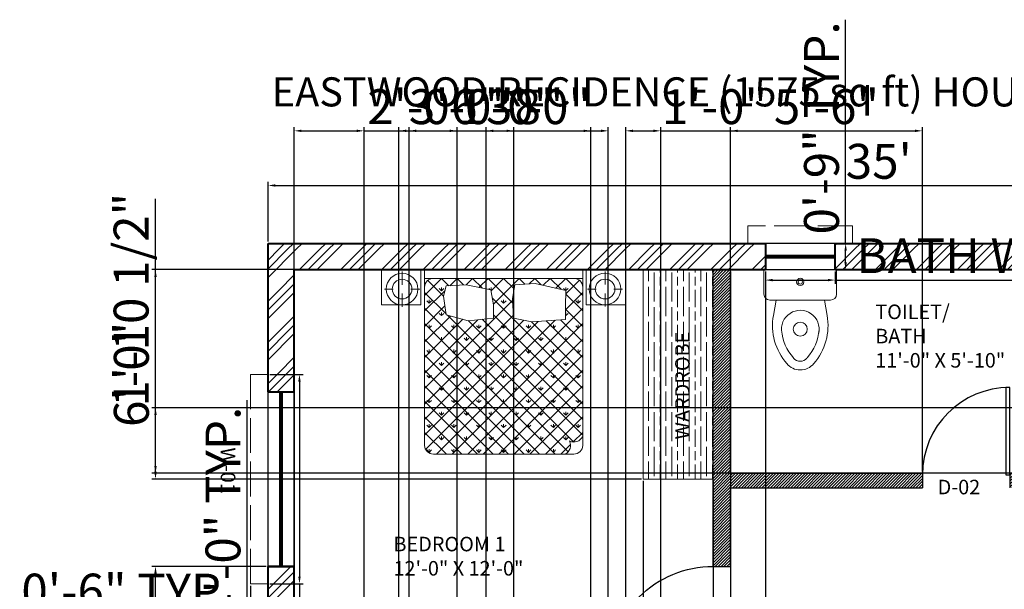
# Model space of a CAD drawing. Units: inches. Extents: x 2386 to 3029, y 792 to 1465.
# Tile 10 of 12: x 2386 to 2724, y 1269 to 1465. Entities that reach past the tile are written whole.
import ezdxf

# ---------------------------------------------------------------- set-up
doc = ezdxf.new("R2010")
doc.units = ezdxf.units.IN
doc.linetypes.add('ACAD_ISO02W100', pattern=[15, 12, -3])
for name, color, linetype, lineweight in [('A-AREA-IDEN', 4, 'Continuous', 25), ('A-DIMS', 1, 'Continuous', 18), ('A-DOOR', 2, 'Continuous', 25), ('A-FLOR-CASE', 6, 'Continuous', 18), ('A-FLOR-CASE-PATT', 9, 'Continuous', 13), ('A-FLOR-FIXT', 9, 'Continuous', 18), ('A-FURN', 6, 'Continuous', 18), ('A-TEXT', 4, 'Continuous', 25), ('A-WALL-EXT', 7, 'Continuous', 40), ('A-WALL-INT', 9, 'Continuous', 30), ('A-WALL-PATT', 9, 'Continuous', 13), ('A-WINDOW', 4, 'Continuous', 25), ('A-WINDOW-OVHD', 4, 'ACAD_ISO02W100', 18)]:
    doc.layers.add(name, color=color, linetype=linetype, lineweight=lineweight)
doc.styles.get("Standard").update_dxf_attribs({"font": 'arial.ttf'})
doc.dimstyles.new('ISO-25', dxfattribs={"dimtxt": 12, "dimasz": 2.5, "dimexe": 1.25, "dimexo": 0.625, "dimtad": 1, "dimlunit": 4, "dimtxsty": 'Standard', "dimcen": 2.5, "dimadec": 0, "dimazin": 0, "dimtfac": 1, "dimtmove": 0, "dimatfit": 3, "dimfxl": 1, "dimarcsym": 0})

# ---------------------------------------------------------------- blocks, each defined once
blk = doc.blocks.new('*X5')
at = {"color": 0}
for p, q in [((0, 0), (0, 0)), ((-707, -141), (-707, -104)), ((-566, 0), (-566, 0)), ((-566, 0), (-566, 0)), ((-283, 0), (-283, 0)), ((-283, 0), (-283, 0)), ((-141, -141), (-141, -104)), ((283, 0), (283, 0)), ((566, 0), (566, 0)), ((707, -135), (707, -104)), ((-707, -141), (-734, -115)), ((-707, -141), (-681, -115)), ((-156, -126), (-168, -115)), ((-141, -141), (-142, -140)), ((-141, -141), (-115, -115)), ((120, -120), (115, -115)), ((699, -134), (681, -115)), ((710, -139), (734, -115)), ((-849, -283), (-875, -256)), ((-849, -283), (-849, -245)), ((-849, -283), (-822, -256)), ((0, -283), (-27, -256)), ((0, -283), (0, -245)), ((0, -283), (27, -256)), ((849, -283), (822, -256)), ((849, -283), (849, -245)), ((849, -283), (875, -256)), ((-707, -424), (-734, -398)), ((-707, -424), (-707, -387)), ((-707, -424), (-681, -398)), ((-116, -399), (-115, -398)), ((707, -424), (703, -420)), ((707, -424), (707, -387)), ((707, -424), (734, -398)), ((-849, -566), (-875, -539)), ((-849, -566), (-849, -528)), ((-849, -566), (-822, -539)), ((-566, -566), (-592, -539)), ((-566, -566), (-566, -528)), ((-566, -566), (-539, -539)), ((-283, -566), (-309, -539)), ((-283, -566), (-283, -528)), ((-283, -566), (-256, -539)), ((0, -566), (-27, -539)), ((0, -566), (0, -528)), ((0, -566), (27, -539)), ((283, -566), (256, -539)), ((283, -566), (283, -528)), ((283, -566), (309, -539)), ((566, -566), (539, -539)), ((566, -566), (566, -528)), ((566, -566), (592, -539)), ((849, -566), (822, -539)), ((849, -566), (849, -528)), ((849, -566), (875, -539)), ((-707, -707), (-707, -670)), ((-424, -707), (-424, -670)), ((-141, -707), (-141, -670)), ((141, -707), (141, -670)), ((424, -707), (424, -670)), ((707, -707), (707, -670)), ((-707, -707), (-734, -681)), ((-707, -707), (-681, -681)), ((-424, -707), (-451, -681)), ((-424, -707), (-398, -681)), ((-141, -707), (-168, -681)), ((-141, -707), (-115, -681)), ((141, -707), (115, -681)), ((141, -707), (168, -681)), ((424, -707), (398, -681)), ((424, -707), (451, -681)), ((707, -707), (681, -681)), ((707, -707), (734, -681)), ((-849, -849), (-875, -822)), ((-849, -849), (-849, -811)), ((-849, -849), (-822, -822)), ((-566, -849), (-592, -822)), ((-566, -849), (-566, -811)), ((-566, -849), (-539, -822)), ((-283, -849), (-309, -822)), ((-283, -849), (-283, -811)), ((-283, -849), (-256, -822)), ((0, -849), (-27, -822)), ((0, -849), (0, -811)), ((0, -849), (27, -822)), ((283, -849), (256, -822)), ((283, -849), (283, -811)), ((283, -849), (309, -822)), ((566, -849), (539, -822)), ((566, -849), (566, -811)), ((566, -849), (592, -822)), ((849, -849), (822, -822)), ((849, -849), (849, -811)), ((849, -849), (875, -822)), ((-707, -990), (-734, -963)), ((-707, -990), (-707, -952)), ((-707, -990), (-681, -963)), ((-424, -990), (-451, -963)), ((-424, -990), (-424, -952)), ((-424, -990), (-398, -963)), ((-141, -990), (-168, -963)), ((-141, -990), (-141, -952)), ((-141, -990), (-115, -963)), ((141, -990), (115, -963)), ((141, -990), (141, -952)), ((141, -990), (168, -963)), ((424, -990), (398, -963)), ((424, -990), (424, -952)), ((424, -990), (451, -963)), ((707, -990), (681, -963)), ((707, -990), (707, -952)), ((707, -990), (734, -963)), ((-849, -1131), (-875, -1105)), ((-849, -1131), (-849, -1094)), ((-849, -1131), (-822, -1105)), ((-566, -1131), (-592, -1105)), ((-566, -1131), (-566, -1094)), ((-566, -1131), (-539, -1105)), ((-283, -1131), (-309, -1105)), ((-283, -1131), (-283, -1094)), ((-283, -1131), (-256, -1105)), ((0, -1131), (-27, -1105)), ((0, -1131), (0, -1094)), ((0, -1131), (27, -1105)), ((283, -1131), (256, -1105)), ((283, -1131), (283, -1094)), ((283, -1131), (309, -1105)), ((566, -1131), (539, -1105)), ((566, -1131), (566, -1094)), ((566, -1131), (592, -1105)), ((849, -1131), (822, -1105)), ((849, -1131), (849, -1094)), ((849, -1131), (875, -1105)), ((-707, -1273), (-734, -1246)), ((-707, -1273), (-707, -1235)), ((-707, -1273), (-681, -1246)), ((-424, -1273), (-451, -1246)), ((-424, -1273), (-424, -1235)), ((-424, -1273), (-398, -1246)), ((-141, -1273), (-168, -1246)), ((-141, -1273), (-141, -1235)), ((-141, -1273), (-115, -1246)), ((141, -1273), (115, -1246)), ((141, -1273), (141, -1235)), ((141, -1273), (168, -1246)), ((424, -1273), (398, -1246)), ((424, -1273), (424, -1235)), ((424, -1273), (451, -1246)), ((707, -1273), (681, -1246)), ((707, -1273), (707, -1235)), ((707, -1273), (734, -1246)), ((-849, -1414), (-875, -1388)), ((-849, -1414), (-849, -1377)), ((-849, -1414), (-822, -1388)), ((-566, -1414), (-592, -1388)), ((-566, -1414), (-566, -1377)), ((-566, -1414), (-539, -1388)), ((-283, -1414), (-309, -1388)), ((-283, -1414), (-283, -1377)), ((-283, -1414), (-256, -1388)), ((0, -1414), (-27, -1388)), ((0, -1414), (0, -1377)), ((0, -1414), (27, -1388)), ((283, -1414), (256, -1388)), ((283, -1414), (283, -1377)), ((283, -1414), (309, -1388)), ((566, -1414), (539, -1388)), ((566, -1414), (566, -1377)), ((566, -1414), (592, -1388)), ((849, -1414), (822, -1388)), ((849, -1414), (849, -1377)), ((849, -1414), (875, -1388)), ((-707, -1556), (-734, -1529)), ((-707, -1556), (-707, -1518)), ((-707, -1556), (-681, -1529)), ((-424, -1556), (-451, -1529)), ((-424, -1556), (-424, -1518)), ((-424, -1556), (-398, -1529)), ((-141, -1556), (-168, -1529)), ((-141, -1556), (-141, -1518)), ((-141, -1556), (-115, -1529)), ((141, -1556), (115, -1529)), ((141, -1556), (141, -1518)), ((141, -1556), (168, -1529)), ((424, -1556), (398, -1529)), ((424, -1556), (424, -1518)), ((424, -1556), (451, -1529)), ((707, -1556), (681, -1529)), ((707, -1556), (707, -1518)), ((707, -1556), (734, -1529)), ((-849, -1697), (-875, -1671)), ((-849, -1697), (-849, -1660)), ((-849, -1697), (-822, -1671)), ((-566, -1697), (-592, -1671)), ((-566, -1697), (-566, -1660)), ((-566, -1697), (-539, -1671)), ((-283, -1697), (-309, -1671)), ((-283, -1697), (-283, -1660)), ((-283, -1697), (-256, -1671)), ((0, -1697), (-27, -1671)), ((0, -1697), (0, -1660)), ((0, -1697), (27, -1671)), ((283, -1697), (256, -1671)), ((283, -1697), (283, -1660)), ((283, -1697), (309, -1671)), ((566, -1697), (539, -1671)), ((566, -1697), (566, -1660)), ((566, -1697), (592, -1671)), ((849, -1697), (822, -1671)), ((849, -1697), (849, -1660)), ((849, -1697), (875, -1671)), ((-707, -1838), (-734, -1812)), ((-707, -1838), (-707, -1801)), ((-707, -1838), (-681, -1812)), ((-424, -1838), (-451, -1812)), ((-424, -1838), (-424, -1801)), ((-424, -1838), (-398, -1812)), ((-141, -1838), (-168, -1812)), ((-141, -1838), (-141, -1801)), ((-141, -1838), (-115, -1812)), ((141, -1838), (115, -1812)), ((141, -1838), (141, -1801)), ((141, -1838), (168, -1812)), ((424, -1838), (398, -1812)), ((424, -1838), (424, -1801)), ((424, -1838), (451, -1812)), ((707, -1838), (681, -1812)), ((707, -1838), (707, -1801)), ((707, -1838), (734, -1812)), ((-849, -1980), (-875, -1953)), ((-849, -1980), (-849, -1942)), ((-849, -1980), (-822, -1953)), ((-566, -1980), (-592, -1953)), ((-566, -1980), (-566, -1942)), ((-566, -1980), (-539, -1953)), ((-283, -1980), (-309, -1953)), ((-283, -1980), (-283, -1942)), ((-283, -1980), (-256, -1953)), ((0, -1980), (-27, -1953)), ((0, -1980), (0, -1942)), ((0, -1980), (27, -1953)), ((283, -1980), (256, -1953)), ((283, -1980), (283, -1942)), ((283, -1980), (309, -1953)), ((566, -1980), (539, -1953)), ((566, -1980), (566, -1942)), ((566, -1980), (592, -1953))]:
    blk.add_line(p, q, dxfattribs=at)
blk = doc.blocks.new('*X4')
at = {"color": 0}
for p, q in [((-900, -193), (-707, 0)), ((-623, -84), (-707, 0)), ((-614, -83), (-530, 0)), ((-457, -74), (-530, 0)), ((-425, -72), (-354, 0)), ((-245, -108), (-354, 0)), ((-278, -101), (-177, 0)), ((103, -280), (-177, 0)), ((-142, -142), (0, 0)), ((-117, -294), (177, 0)), ((120, -120), (0, 0)), ((241, -64), (177, 0)), ((292, -61), (354, 0)), ((426, -72), (354, 0)), ((452, -78), (530, 0)), ((654, -123), (530, 0)), ((596, -111), (707, 0)), ((900, -193), (707, 0)), ((-683, -201), (-862, -22)), ((708, -175), (862, -22)), ((-900, -370), (-667, -137)), ((-656, -405), (-900, -161)), ((703, -358), (900, -161)), ((900, -370), (708, -178)), ((-900, -1254), (101, -252)), ((-900, -546), (-668, -314)), ((900, -1254), (-128, -225)), ((735, -1973), (-900, -337)), ((-900, -1430), (112, -418)), ((-900, -723), (-605, -429)), ((-763, -2000), (900, -337)), ((801, -1862), (-641, -419)), ((900, -1430), (-116, -415)), ((900, -546), (703, -349)), ((-900, -900), (-465, -465)), ((-900, -1077), (-293, -470)), ((-900, -1607), (231, -476)), ((-900, -1784), (394, -489)), ((586, -2000), (-900, -514)), ((-888, -1948), (586, -475)), ((-586, -2000), (900, -514)), ((900, -1784), (-404, -480)), ((900, -1607), (-243, -465)), ((900, -1077), (317, -494)), ((900, -900), (483, -483)), ((900, -723), (647, -470)), ((409, -2000), (-900, -691)), ((-409, -2000), (900, -691)), ((232, -2000), (-900, -868)), ((-232, -2000), (900, -868)), ((55, -2000), (-900, -1045)), ((-55, -2000), (900, -1045)), ((-121, -2000), (-900, -1221)), ((121, -2000), (900, -1221)), ((-298, -2000), (-900, -1398)), ((298, -2000), (900, -1398)), ((-475, -2000), (-900, -1575)), ((475, -2000), (900, -1575)), ((-652, -2000), (-900, -1752)), ((790, -1861), (900, -1752)), ((652, -2000), (761, -1890)), ((-835, -1994), (-894, -1935))]:
    blk.add_line(p, q, dxfattribs=at)
blk = doc.blocks.new('A$C190D2546')
at = {"layer": 'A-FURN'}
for p, q in [((285, 1928), (285, 2078)), ((541, 2100), (2341, 2100)), ((541, 1881), (541, 2100)), ((2341, 1881), (2341, 2100)), ((2596, 1929), (2596, 2079)), ((2341, 2000), (541, 2000)), ((185, 1878), (85, 1878)), ((285, 1828), (285, 1678)), ((385, 1878), (485, 1878)), ((2496, 1879), (2396, 1879)), ((2596, 1829), (2596, 1679)), ((2696, 1879), (2796, 1879))]:
    blk.add_line(p, q, dxfattribs=at)
for points in [[(500, 2101), (500, 1701), (50, 1701), (50, 2101)], [(2382, 2101), (2382, 1701), (2832, 1701), (2832, 2101)], [(787, 1584), (758, 1799), (787, 1914), (1016, 1928), (1296, 1871), (1325, 1699), (1325, 1548), (1038, 1519)], [(1555, 1548), (1541, 1771), (1569, 1928), (1799, 1943), (2151, 1864), (2144, 1685), (2144, 1534), (1763, 1505)]]:
    blk.add_lwpolyline(points, close=True, dxfattribs=at)
blk.add_lwpolyline([(641, 2000), (2241, 2000, -0.414214), (2341, 1900), (2341, 100, -0.414214), (2241, 0), (641, 0, -0.414214), (541, 100), (541, 1900, -0.414214)], format="xyb", close=True, dxfattribs=at)
for centre, radius in [((285, 1878), 180), ((2596, 1879), 180), ((285, 1878), 112), ((2596, 1879), 112)]:
    blk.add_circle(centre, radius, dxfattribs=at)
for centre, start, end in [((2091, 100), 296.5651, 26.5651), ((2241, 250), 243.4349, 333.4349)]:
    blk.add_arc(centre, 112, start, end, dxfattribs=at)
for name in ['*X4', '*X5']:
    blk.add_blockref(name, (1441, 2000), dxfattribs=at)
blk = doc.blocks.new('*U13')
for p, q in [((0, 0), (0, 6)), ((40, 0), (40, 6))]:
    blk.add_line(p, q)
blk.add_lwpolyline([(0, 0), (0, -40), (1.75, -40), (1.75, 0)], close=True)
blk.add_arc((0, 0), 40, 270, 0)
blk = doc.blocks.new('*U3')
for p, q in [((0, 0), (0, -6)), ((-40, 0), (-40, -6))]:
    blk.add_line(p, q)
blk.add_lwpolyline([(0, 0), (0, 40), (-1.75, 40), (-1.75, 0)], close=True)
blk.add_arc((0, 0), 40, 90, 180)
blk = doc.blocks.new('*D21')
at = {"layer": 'A-DIMS', "color": 0, "lineweight": -2, "transparency": 16777216}
for p, q in [((2471.19, 1388.57), (2471.19, 1409.12)), ((2891.19, 1388.57), (2891.19, 1409.12)), ((2473.69, 1407.87), (2888.69, 1407.87))]:
    blk.add_line(p, q, dxfattribs=at)
at = {"layer": 'A-DIMS', "color": 0, "transparency": 16777216}
for points in [[(2473.69, 1408.28), (2473.69, 1407.45), (2471.19, 1407.87)], [(2888.69, 1408.28), (2888.69, 1407.45), (2891.19, 1407.87)]]:
    blk.add_solid(points, dxfattribs=at)
at = {"layer": 'Defpoints', "color": 0, "transparency": 16777216}
for p in [(2891.19, 1407.87), (2471.19, 1387.95), (2891.19, 1387.95)]:
    blk.add_point(p, dxfattribs=at)
at = {"layer": 'A-DIMS', "color": 0, "transparency": 16777216, "insert": (2681.19, 1414.62), "char_height": 12, "attachment_point": 5}
blk.add_mtext("35'", dxfattribs=at)
blk = doc.blocks.new('WC-FLOOR-MOUNT')
for p, q in [((34.48, 25), (26.06, 25)), ((18.75, 21.75), (23.99, 20.83)), ((24, 22.94), (24, 2.06)), ((18.75, 3.25), (23.99, 4.16)), ((34.48, 0), (26.06, 0))]:
    blk.add_line(p, q)
for centre, radius in [((14.02, 12.49), 2.41), ((30.25, 12.5), 1.25), ((30.25, 12.5), 0.75)]:
    blk.add_circle(centre, radius)
for centre, radius, start, end in [((26.06, 22.94), 2.06, 90, 180), ((15.32, 2.04), 20, 80.1061, 131.065), ((6, 12.5), 6, 129.5742, 180), ((15.32, 2.04), 17, 95.686, 131.065), ((14.02, 12.49), 6.48, 257.3713, 100.6839), ((6, 12.5), 3, 129.5742, 180), ((6, 12.5), 6, 180, 230.4258), ((6, 12.5), 3, 180, 230.4258), ((15.32, 22.95), 20, 228.935, 279.8939), ((15.32, 22.95), 17, 228.935, 265.0633), ((26.06, 2.06), 2.06, 180, 270)]:
    blk.add_arc(centre, radius, start, end)
blk = doc.blocks.new('WINDOW-60IN')
for p, q in [((0, 0), (0, 60)), ((0, 60), (9, 60)), ((4, 60), (4, 0)), ((4, 59.5), (5, 59.5)), ((4.5, 59.5), (4.5, 0.5)), ((5, 60), (5, 0)), ((9, 60), (9, 0)), ((0, 0), (9, 0)), ((5, 0.5), (4, 0.5))]:
    blk.add_line(p, q)
blk = doc.blocks.new('WINDOW-HOOD-60IN')
for p, q in [((0, 72), (6, 72)), ((6, 72), (6, 0)), ((0, 0), (6, 0))]:
    blk.add_line(p, q)
blk = doc.blocks.new('WINDOW-24IN')
for p, q in [((24, 9), (0, 9)), ((0, 0), (0, 9)), ((24, 0), (24, 9)), ((0, 5), (24, 5)), ((0, 4), (24, 4)), ((0.5, 5), (0.5, 4)), ((0.5, 4.5), (23.5, 4.5)), ((23.5, 4), (23.5, 5)), ((0, 0), (24, 0))]:
    blk.add_line(p, q)
blk = doc.blocks.new('WINDOW-HOOD-24IN')
for p, q in [((36, 6), (0, 6)), ((0, 0), (0, 6)), ((36, 0), (36, 6))]:
    blk.add_line(p, q)
blk = doc.blocks.new('*D38')
at = {"layer": 'A-DIMS', "color": 0, "lineweight": -2, "transparency": 16777216}
for p, q in [((2471.82, 1342.95), (2483.24, 1342.95)), ((2481.99, 1340.45), (2481.99, 1273.45)), ((2471.82, 1270.95), (2483.24, 1270.95)), ((2481.99, 1270.95), (2481.99, 1095.04))]:
    blk.add_line(p, q, dxfattribs=at)
at = {"layer": 'A-DIMS', "color": 0, "transparency": 16777216}
for points in [[(2481.57, 1340.45), (2482.41, 1340.45), (2481.99, 1342.95)], [(2481.57, 1273.45), (2482.41, 1273.45), (2481.99, 1270.95)]]:
    blk.add_solid(points, dxfattribs=at)
at = {"layer": 'Defpoints', "color": 0, "transparency": 16777216}
for p in [(2471.19, 1342.95), (2471.19, 1270.95), (2481.99, 1270.95)]:
    blk.add_point(p, dxfattribs=at)
at = {"layer": 'A-DIMS', "color": 0, "transparency": 16777216, "insert": (2475.16, 1181.74), "char_height": 12, "attachment_point": 5, "rotation": 90}
blk.add_mtext('HOOD W-01 6\'-0" TYP.', dxfattribs=at)
blk = doc.blocks.new('*D39')
at = {"layer": 'A-DIMS', "color": 0, "lineweight": -2, "transparency": 16777216}
for p, q in [((2465.19, 1270.32), (2465.19, 1258.9)), ((2471.19, 1270.32), (2471.19, 1258.9)), ((2462.69, 1260.15), (2385.79, 1260.15)), ((2471.19, 1260.15), (2465.19, 1260.15)), ((2473.69, 1260.15), (2476.19, 1260.15))]:
    blk.add_line(p, q, dxfattribs=at)
at = {"layer": 'A-DIMS', "color": 0, "transparency": 16777216}
for points in [[(2462.69, 1260.56), (2462.69, 1259.73), (2465.19, 1260.15)], [(2473.69, 1260.56), (2473.69, 1259.73), (2471.19, 1260.15)]]:
    blk.add_solid(points, dxfattribs=at)
at = {"layer": 'Defpoints', "color": 0, "transparency": 16777216}
for p in [(2465.19, 1270.95), (2471.19, 1270.95), (2465.19, 1260.15)]:
    blk.add_point(p, dxfattribs=at)
at = {"layer": 'A-DIMS', "color": 0, "transparency": 16777216, "insert": (2422.99, 1266.9), "char_height": 12, "attachment_point": 5}
blk.add_mtext('0\'-6" TYP.', dxfattribs=at)
blk = doc.blocks.new('*D40')
at = {"layer": 'A-DIMS', "color": 0, "lineweight": -2, "transparency": 16777216}
for p, q in [((2463.99, 1211.95), (2463.99, 1334.04)), ((2470.57, 1211.95), (2462.74, 1211.95)), ((2463.99, 1166.45), (2463.99, 1209.45)), ((2470.57, 1163.95), (2462.74, 1163.95))]:
    blk.add_line(p, q, dxfattribs=at)
at = {"layer": 'A-DIMS', "color": 0, "transparency": 16777216}
for points in [[(2463.57, 1209.45), (2464.41, 1209.45), (2463.99, 1211.95)], [(2463.57, 1166.45), (2464.41, 1166.45), (2463.99, 1163.95)]]:
    blk.add_solid(points, dxfattribs=at)
at = {"layer": 'Defpoints', "color": 0, "transparency": 16777216}
for p in [(2463.99, 1211.95), (2471.19, 1211.95), (2471.19, 1163.95)]:
    blk.add_point(p, dxfattribs=at)
at = {"layer": 'A-DIMS', "color": 0, "transparency": 16777216, "insert": (2457.24, 1274.25), "char_height": 12, "attachment_point": 5, "rotation": 90}
blk.add_mtext('W-02 4\'-0" TYP.', dxfattribs=at)
blk = doc.blocks.new('*D48')
at = {"layer": 'A-DIMS', "color": 0, "lineweight": -2, "transparency": 16777216}
for p, q in [((2642.19, 1378.32), (2642.19, 1374.1)), ((2666.19, 1378.32), (2666.19, 1374.1)), ((2644.69, 1375.35), (2663.69, 1375.35)), ((2666.19, 1375.35), (2870.13, 1375.35))]:
    blk.add_line(p, q, dxfattribs=at)
at = {"layer": 'A-DIMS', "color": 0, "transparency": 16777216}
for points in [[(2644.69, 1375.76), (2644.69, 1374.93), (2642.19, 1375.35)], [(2663.69, 1375.76), (2663.69, 1374.93), (2666.19, 1375.35)]]:
    blk.add_solid(points, dxfattribs=at)
at = {"layer": 'Defpoints', "color": 0, "transparency": 16777216}
for p in [(2642.19, 1378.95), (2666.19, 1378.95), (2666.19, 1375.35)]:
    blk.add_point(p, dxfattribs=at)
at = {"layer": 'A-DIMS', "color": 0, "transparency": 16777216, "insert": (2769.41, 1382.18), "char_height": 12, "attachment_point": 5}
blk.add_mtext('BATH WINDOW 2\'-0" TYP.', dxfattribs=at)
blk = doc.blocks.new('*D49')
at = {"layer": 'A-DIMS', "color": 0, "lineweight": -2, "transparency": 16777216}
for p, q in [((2669.79, 1387.95), (2669.79, 1464.84)), ((2666.82, 1387.95), (2671.04, 1387.95)), ((2669.79, 1381.45), (2669.79, 1385.45)), ((2666.82, 1378.95), (2671.04, 1378.95))]:
    blk.add_line(p, q, dxfattribs=at)
at = {"layer": 'A-DIMS', "color": 0, "transparency": 16777216}
for points in [[(2669.37, 1385.45), (2670.21, 1385.45), (2669.79, 1387.95)], [(2669.37, 1381.45), (2670.21, 1381.45), (2669.79, 1378.95)]]:
    blk.add_solid(points, dxfattribs=at)
at = {"layer": 'Defpoints', "color": 0, "transparency": 16777216}
for p in [(2666.19, 1387.95), (2669.79, 1387.95), (2666.19, 1378.95)]:
    blk.add_point(p, dxfattribs=at)
at = {"layer": 'A-DIMS', "color": 0, "transparency": 16777216, "insert": (2663.04, 1427.65), "char_height": 12, "attachment_point": 5, "rotation": 90}
blk.add_mtext('0\'-9" TYP.', dxfattribs=at)
blk = doc.blocks.new('*D57')
at = {"layer": 'A-DIMS', "color": 0, "lineweight": -2, "transparency": 16777216}
for p, q in [((2546.19, 1008.57), (2546.19, 1427.9)), ((2548.69, 1426.65), (2579.69, 1426.65)), ((2582.19, 1008.57), (2582.19, 1427.9))]:
    blk.add_line(p, q, dxfattribs=at)
at = {"layer": 'A-DIMS', "color": 0, "transparency": 16777216}
for points in [[(2548.69, 1427.06), (2548.69, 1426.23), (2546.19, 1426.65)], [(2579.69, 1427.06), (2579.69, 1426.23), (2582.19, 1426.65)]]:
    blk.add_solid(points, dxfattribs=at)
at = {"layer": 'Defpoints', "color": 0, "transparency": 16777216}
for p in [(2582.19, 1426.65), (2546.19, 1007.95), (2582.19, 1007.95)]:
    blk.add_point(p, dxfattribs=at)
at = {"layer": 'A-DIMS', "color": 0, "transparency": 16777216, "insert": (2564.19, 1433.4), "char_height": 12, "attachment_point": 5}
blk.add_mtext('3\'-0"', dxfattribs=at)
blk = doc.blocks.new('*D65')
at = {"layer": 'A-DIMS', "color": 0, "lineweight": -2, "transparency": 16777216}
for p, q in [((2470.57, 1276.95), (2431.24, 1276.95)), ((2432.49, 1214.45), (2432.49, 1274.45)), ((2470.57, 1211.95), (2431.24, 1211.95))]:
    blk.add_line(p, q, dxfattribs=at)
at = {"layer": 'A-DIMS', "color": 0, "transparency": 16777216}
for points in [[(2432.07, 1274.45), (2432.91, 1274.45), (2432.49, 1276.95)], [(2432.07, 1214.45), (2432.91, 1214.45), (2432.49, 1211.95)]]:
    blk.add_solid(points, dxfattribs=at)
at = {"layer": 'Defpoints', "color": 0, "transparency": 16777216}
for p in [(2432.49, 1276.95), (2471.19, 1276.95), (2471.19, 1211.95)]:
    blk.add_point(p, dxfattribs=at)
at = {"layer": 'A-DIMS', "color": 0, "transparency": 16777216, "insert": (2425.76, 1244.45), "char_height": 12, "attachment_point": 5, "rotation": 90}
blk.add_mtext('5\'-5"', dxfattribs=at)
blk = doc.blocks.new('*D66')
at = {"layer": 'A-DIMS', "color": 0, "lineweight": -2, "transparency": 16777216}
for p, q in [((2630.19, 1378.32), (2630.19, 808)), ((2642.19, 1378.32), (2642.19, 808)), ((2632.69, 809.25), (2639.69, 809.25)), ((2642.19, 809.25), (2676.71, 809.25))]:
    blk.add_line(p, q, dxfattribs=at)
at = {"layer": 'A-DIMS', "color": 0, "transparency": 16777216}
for points in [[(2632.69, 809.66), (2632.69, 808.83), (2630.19, 809.25)], [(2639.69, 809.66), (2639.69, 808.83), (2642.19, 809.25)]]:
    blk.add_solid(points, dxfattribs=at)
at = {"layer": 'Defpoints', "color": 0, "transparency": 16777216}
for p in [(2630.19, 1378.95), (2642.19, 1378.95), (2642.19, 809.25)]:
    blk.add_point(p, dxfattribs=at)
at = {"layer": 'A-DIMS', "color": 0, "transparency": 16777216, "insert": (2660.7, 816), "char_height": 12, "attachment_point": 5}
blk.add_mtext('1\'-0"', dxfattribs=at)
blk = doc.blocks.new('*D73')
at = {"layer": 'A-DIMS', "color": 0, "lineweight": -2, "transparency": 16777216}
for p, q in [((2519.68, 889.97), (2519.68, 1427.9)), ((2522.18, 1426.65), (2553.18, 1426.65)), ((2555.68, 889.97), (2555.68, 1427.9))]:
    blk.add_line(p, q, dxfattribs=at)
at = {"layer": 'A-DIMS', "color": 0, "transparency": 16777216}
for points in [[(2522.18, 1427.06), (2522.18, 1426.23), (2519.68, 1426.65)], [(2553.18, 1427.06), (2553.18, 1426.23), (2555.68, 1426.65)]]:
    blk.add_solid(points, dxfattribs=at)
at = {"layer": 'Defpoints', "color": 0, "transparency": 16777216}
for p in [(2555.68, 1426.65), (2519.68, 889.35), (2555.68, 889.35)]:
    blk.add_point(p, dxfattribs=at)
at = {"layer": 'A-DIMS', "color": 0, "transparency": 16777216, "insert": (2537.68, 1433.4), "char_height": 12, "attachment_point": 5}
blk.add_mtext('3\'-0"', dxfattribs=at)
blk = doc.blocks.new('*D78')
at = {"layer": 'A-DIMS', "color": 0, "lineweight": -2, "transparency": 16777216}
for p, q in [((2516.19, 1054.57), (2516.19, 1427.9)), ((2518.69, 1426.65), (2533.69, 1426.65)), ((2536.19, 1044.57), (2536.19, 1427.9)), ((2536.19, 1426.65), (2570.71, 1426.65))]:
    blk.add_line(p, q, dxfattribs=at)
at = {"layer": 'A-DIMS', "color": 0, "transparency": 16777216}
for points in [[(2518.69, 1427.06), (2518.69, 1426.23), (2516.19, 1426.65)], [(2533.69, 1427.06), (2533.69, 1426.23), (2536.19, 1426.65)]]:
    blk.add_solid(points, dxfattribs=at)
at = {"layer": 'Defpoints', "color": 0, "transparency": 16777216}
for p in [(2536.19, 1426.65), (2516.19, 1053.95), (2536.19, 1043.95)]:
    blk.add_point(p, dxfattribs=at)
at = {"layer": 'A-DIMS', "color": 0, "transparency": 16777216, "insert": (2554.7, 1433.4), "char_height": 12, "attachment_point": 5}
blk.add_mtext('1\'-8"', dxfattribs=at)
blk = doc.blocks.new('*D82')
at = {"layer": 'A-DIMS', "color": 0, "lineweight": -2, "transparency": 16777216}
for p, q in [((2600.19, 1306.32), (2600.19, 808)), ((2624.19, 1306.32), (2624.19, 808)), ((2602.69, 809.25), (2621.69, 809.25)), ((2624.19, 809.25), (2660.04, 809.25))]:
    blk.add_line(p, q, dxfattribs=at)
at = {"layer": 'A-DIMS', "color": 0, "transparency": 16777216}
for points in [[(2602.69, 809.66), (2602.69, 808.83), (2600.19, 809.25)], [(2621.69, 809.66), (2621.69, 808.83), (2624.19, 809.25)]]:
    blk.add_solid(points, dxfattribs=at)
at = {"layer": 'Defpoints', "color": 0, "transparency": 16777216}
for p in [(2600.19, 1306.95), (2624.19, 1306.95), (2624.19, 809.25)]:
    blk.add_point(p, dxfattribs=at)
at = {"layer": 'A-DIMS', "color": 0, "transparency": 16777216, "insert": (2643.37, 816), "char_height": 12, "attachment_point": 5}
blk.add_mtext('2\'-0"', dxfattribs=at)
blk = doc.blocks.new('*D83')
at = {"layer": 'A-DIMS', "color": 0, "lineweight": -2, "transparency": 16777216}
for p, q in [((2599.57, 1378.95), (2431.24, 1378.95)), ((2432.49, 1309.45), (2432.49, 1376.45)), ((2599.57, 1306.95), (2431.24, 1306.95))]:
    blk.add_line(p, q, dxfattribs=at)
at = {"layer": 'A-DIMS', "color": 0, "transparency": 16777216}
for points in [[(2432.07, 1376.45), (2432.91, 1376.45), (2432.49, 1378.95)], [(2432.07, 1309.45), (2432.91, 1309.45), (2432.49, 1306.95)]]:
    blk.add_solid(points, dxfattribs=at)
at = {"layer": 'Defpoints', "color": 0, "transparency": 16777216}
for p in [(2432.49, 1378.95), (2600.19, 1378.95), (2600.19, 1306.95)]:
    blk.add_point(p, dxfattribs=at)
at = {"layer": 'A-DIMS', "color": 0, "transparency": 16777216, "insert": (2425.74, 1342.95), "char_height": 12, "attachment_point": 5, "rotation": 90}
blk.add_mtext('6\'-0"', dxfattribs=at)
blk = doc.blocks.new('*D87')
at = {"layer": 'A-DIMS', "color": 0, "lineweight": -2, "transparency": 16777216}
for p, q in [((2594.19, 921.57), (2594.19, 1427.9)), ((2596.69, 1426.65), (2603.69, 1426.65)), ((2606.19, 921.57), (2606.19, 1427.9)), ((2606.19, 1426.65), (2640.71, 1426.65))]:
    blk.add_line(p, q, dxfattribs=at)
at = {"layer": 'A-DIMS', "color": 0, "transparency": 16777216}
for points in [[(2596.69, 1427.06), (2596.69, 1426.23), (2594.19, 1426.65)], [(2603.69, 1427.06), (2603.69, 1426.23), (2606.19, 1426.65)]]:
    blk.add_solid(points, dxfattribs=at)
at = {"layer": 'Defpoints', "color": 0, "transparency": 16777216}
for p in [(2606.19, 1426.65), (2594.19, 920.95), (2606.19, 920.95)]:
    blk.add_point(p, dxfattribs=at)
at = {"layer": 'A-DIMS', "color": 0, "transparency": 16777216, "insert": (2624.7, 1433.4), "char_height": 12, "attachment_point": 5}
blk.add_mtext('1\'-0"', dxfattribs=at)
blk = doc.blocks.new('*D89')
at = {"layer": 'A-DIMS', "color": 0, "lineweight": -2, "transparency": 16777216}
for p, q in [((2432.49, 1331.45), (2432.49, 1403.25)), ((2881.57, 1331.45), (2431.24, 1331.45)), ((2432.49, 1311.45), (2432.49, 1328.95)), ((2881.57, 1308.95), (2431.24, 1308.95))]:
    blk.add_line(p, q, dxfattribs=at)
at = {"layer": 'A-DIMS', "color": 0, "transparency": 16777216}
for points in [[(2432.07, 1328.95), (2432.91, 1328.95), (2432.49, 1331.45)], [(2432.07, 1311.45), (2432.91, 1311.45), (2432.49, 1308.95)]]:
    blk.add_solid(points, dxfattribs=at)
at = {"layer": 'Defpoints', "color": 0, "transparency": 16777216}
for p in [(2432.49, 1331.45), (2882.19, 1331.45), (2882.19, 1308.95)]:
    blk.add_point(p, dxfattribs=at)
at = {"layer": 'A-DIMS', "color": 0, "transparency": 16777216, "insert": (2425.66, 1368.6), "char_height": 12, "attachment_point": 5, "rotation": 90}
blk.add_mtext('1\'-10 1/2"', dxfattribs=at)
blk = doc.blocks.new('*D91')
at = {"layer": 'A-DIMS', "color": 0, "lineweight": -2, "transparency": 16777216}
for p, q in [((2630.19, 1309.57), (2630.19, 1427.9)), ((2632.69, 1426.65), (2693.69, 1426.65)), ((2696.19, 1309.57), (2696.19, 1427.9))]:
    blk.add_line(p, q, dxfattribs=at)
at = {"layer": 'A-DIMS', "color": 0, "transparency": 16777216}
for points in [[(2632.69, 1427.06), (2632.69, 1426.23), (2630.19, 1426.65)], [(2693.69, 1427.06), (2693.69, 1426.23), (2696.19, 1426.65)]]:
    blk.add_solid(points, dxfattribs=at)
at = {"layer": 'Defpoints', "color": 0, "transparency": 16777216}
for p in [(2696.19, 1426.65), (2630.19, 1308.95), (2696.19, 1308.95)]:
    blk.add_point(p, dxfattribs=at)
at = {"layer": 'A-DIMS', "color": 0, "transparency": 16777216, "insert": (2663.19, 1433.4), "char_height": 12, "attachment_point": 5}
blk.add_mtext('5\'-6"', dxfattribs=at)
blk = doc.blocks.new('*D95')
at = {"layer": 'A-DIMS', "color": 0, "lineweight": -2, "transparency": 16777216}
for p, q in [((2480.19, 1146.57), (2480.19, 1427.9)), ((2482.69, 1426.65), (2501.69, 1426.65)), ((2504.19, 1146.57), (2504.19, 1427.9)), ((2504.19, 1426.65), (2540.04, 1426.65))]:
    blk.add_line(p, q, dxfattribs=at)
at = {"layer": 'A-DIMS', "color": 0, "transparency": 16777216}
for points in [[(2482.69, 1427.06), (2482.69, 1426.23), (2480.19, 1426.65)], [(2501.69, 1427.06), (2501.69, 1426.23), (2504.19, 1426.65)]]:
    blk.add_solid(points, dxfattribs=at)
at = {"layer": 'Defpoints', "color": 0, "transparency": 16777216}
for p in [(2504.19, 1426.65), (2480.19, 1145.95), (2504.19, 1145.95)]:
    blk.add_point(p, dxfattribs=at)
at = {"layer": 'A-DIMS', "color": 0, "transparency": 16777216, "insert": (2523.37, 1433.4), "char_height": 12, "attachment_point": 5}
blk.add_mtext('2\'-0"', dxfattribs=at)
blk = doc.blocks.new('*D96')
at = {"layer": 'A-DIMS', "color": 0, "lineweight": -2, "transparency": 16777216}
for p, q in [((2516.19, 893.57), (2516.19, 1427.9)), ((2518.69, 1426.65), (2585.69, 1426.65)), ((2588.19, 893.57), (2588.19, 1427.9))]:
    blk.add_line(p, q, dxfattribs=at)
at = {"layer": 'A-DIMS', "color": 0, "transparency": 16777216}
for points in [[(2518.69, 1427.06), (2518.69, 1426.23), (2516.19, 1426.65)], [(2585.69, 1427.06), (2585.69, 1426.23), (2588.19, 1426.65)]]:
    blk.add_solid(points, dxfattribs=at)
at = {"layer": 'Defpoints', "color": 0, "transparency": 16777216}
for p in [(2588.19, 1426.65), (2516.19, 892.95), (2588.19, 892.95)]:
    blk.add_point(p, dxfattribs=at)
at = {"layer": 'A-DIMS', "color": 0, "transparency": 16777216, "insert": (2552.19, 1433.4), "char_height": 12, "attachment_point": 5}
blk.add_mtext('6\'-0"', dxfattribs=at)

msp = doc.modelspace()

# ---------------------------------------------------------------- hatches: boundary and pattern name
at = {"layer": 'A-FLOR-CASE-PATT'}
h = msp.add_hatch(dxfattribs=at)
h.set_pattern_fill('GOST_WOOD', color=256)
h.paths.add_polyline_path([(2882.19, 1303.948), (2810.19, 1303.948), (2810.19, 1285.948), (2882.19, 1285.948)])
h.paths.add_polyline_path([(2624.19, 1378.948), (2600.19, 1378.948), (2600.19, 1306.948), (2624.19, 1306.948)])
h.paths.add_polyline_path([(2823.021, 1289.11), (2866.657, 1289.11), (2866.657, 1299.414), (2823.021, 1299.414)], flags=24)
h.paths.add_polyline_path([(2618.821, 1319.237), (2618.821, 1362.873), (2608.517, 1362.873), (2608.517, 1319.237)], flags=24)
at = {"layer": 'A-WALL-PATT'}
h = msp.add_hatch(dxfattribs=at)
h.set_pattern_fill('GOST_GROUND', color=256)
h.paths.add_polyline_path([(2480.19, 1276.948), (2471.19, 1276.948), (2471.19, 1211.948), (2480.19, 1211.948)])
h.paths.add_polyline_path([(2480.19, 1378.948), (2510.19, 1378.948), (2510.19, 1378.969), (2523.779, 1378.969), (2580.602, 1378.959), (2580.602, 1378.969), (2594.19, 1378.969), (2642.19, 1378.948), (2642.19, 1387.948), (2471.19, 1387.948), (2471.19, 1336.948), (2480.19, 1336.948)])
h.paths.add_polyline_path([(2891.19, 1387.948), (2666.19, 1387.948), (2666.19, 1378.948), (2882.19, 1378.948), (2882.19, 1355.948), (2891.19, 1355.948)])
h.paths.add_polyline_path([(2891.19, 1331.948), (2882.19, 1331.948), (2882.19, 1331.449), (2882.19, 1261.948), (2891.19, 1261.948)])
h.paths.add_polyline_path([(2891.19, 1201.948), (2882.19, 1201.948), (2882.19, 1189.948), (2882.19, 1159.948), (2882.19, 1117.948), (2891.19, 1117.948)])
h.paths.add_polyline_path([(2891.19, 1057.948), (2882.19, 1057.948), (2882.19, 856.948), (2882.19, 847.948), (2891.19, 847.948)])
h.paths.add_polyline_path([(2594.19, 856.948), (2558.19, 856.948), (2558.19, 847.948), (2594.19, 847.948)])
h.paths.add_polyline_path([(2510.19, 856.948), (2480.19, 856.948), (2480.19, 905.448), (2471.19, 905.448), (2471.19, 847.948), (2510.19, 847.948)])
h.paths.add_polyline_path([(2480.19, 1007.948), (2471.19, 1007.948), (2471.19, 953.448), (2480.19, 953.448)])
h.paths.add_polyline_path([(2480.19, 1103.948), (2471.19, 1103.948), (2471.19, 1043.948), (2480.19, 1043.948)])
h = msp.add_hatch(dxfattribs=at)
h.set_pattern_fill('JIS_WOOD', color=256)
h.paths.add_polyline_path([(2624.19, 1229.948), (2624.19, 1145.948), (2618.19, 1145.948), (2618.19, 1140.548), (2618.19, 1139.948), (2630.19, 1139.948), (2630.19, 1240.948), (2624.19, 1240.948), (2624.19, 1234.948), (2480.19, 1234.948), (2480.19, 1229.948)])
h.paths.add_polyline_path([(2582.19, 1139.948), (2582.19, 1145.948), (2480.19, 1145.948), (2480.19, 1139.948)], flags=17)
h.paths.add_polyline_path([(2480.19, 1007.948), (2480.19, 1001.948), (2546.19, 1001.948), (2546.19, 1007.348), (2546.19, 1007.948)])
h.paths.add_polyline_path([(2594.19, 1007.948), (2582.19, 1007.948), (2582.19, 1001.948), (2588.19, 1001.948), (2588.19, 856.948), (2594.19, 856.948), (2594.19, 914.948), (2606.19, 914.948), (2606.19, 920.948), (2594.19, 920.948)])
h.paths.add_polyline_path([(2738.19, 1015.948), (2882.19, 1015.948), (2882.19, 1021.948), (2738.19, 1021.948), (2738.19, 1111.948), (2732.19, 1111.948), (2732.19, 920.948), (2720.19, 920.948), (2720.19, 914.948), (2732.19, 914.948), (2732.19, 856.948), (2738.19, 856.948)])
h.paths.add_polyline_path([(2660.19, 914.948), (2660.19, 920.948), (2648.19, 920.948), (2648.19, 914.948)])
h.paths.add_polyline_path([(2738.19, 1159.948), (2738.19, 1165.948), (2737.59, 1165.948), (2732.19, 1165.948), (2732.19, 1147.948), (2737.59, 1147.948), (2738.19, 1147.948), (2738.19, 1153.948), (2882.19, 1153.948), (2882.19, 1159.948)])
h.paths.add_polyline_path([(2732.19, 1201.948), (2738.19, 1201.948), (2738.19, 1303.948), (2774.19, 1303.948), (2774.19, 1308.948), (2768.19, 1308.948), (2768.19, 1378.948), (2762.19, 1378.948), (2762.19, 1308.948), (2726.19, 1308.948), (2726.19, 1303.948), (2732.19, 1303.948)])
h.paths.add_polyline_path([(2696.19, 1303.948), (2696.19, 1308.948), (2630.19, 1308.948), (2630.19, 1378.948), (2624.19, 1378.948), (2624.19, 1276.948), (2630.19, 1276.948), (2630.19, 1303.948)])

# ---------------------------------------------------------------- linework, layer by layer
at = {"layer": 'A-FLOR-CASE'}
msp.add_lwpolyline([(2624.19, 1306.948), (2600.19, 1306.948), (2600.19, 1378.948)], dxfattribs=at)
at = {"layer": 'A-FLOR-FIXT'}
msp.add_line((2641.692, 1378.948), (2666.689, 1378.948), dxfattribs=at)
at = {"layer": 'A-WALL-EXT'}
for p, q in [((2471.19, 1387.948), (2642.19, 1387.948)), ((2471.19, 1336.948), (2471.19, 1387.948)), ((2642.19, 1387.948), (2642.19, 1378.948)), ((2666.19, 1387.948), (2891.19, 1387.948)), ((2666.19, 1378.948), (2666.19, 1387.948)), ((2480.19, 1378.948), (2642.19, 1378.948)), ((2480.19, 1336.948), (2480.19, 1378.948)), ((2666.19, 1378.948), (2882.19, 1378.948)), ((2471.19, 1336.948), (2480.19, 1336.948)), ((2471.19, 1336.948), (2480.19, 1336.948)), ((2471.19, 1211.948), (2471.19, 1276.948)), ((2471.19, 1276.948), (2480.19, 1276.948)), ((2480.19, 1276.948), (2471.19, 1276.948)), ((2480.19, 1211.948), (2480.19, 1276.948))]:
    msp.add_line(p, q, dxfattribs=at)
at = {"layer": 'A-WALL-INT'}
for p, q in [((2624.19, 1276.948), (2624.19, 1378.948)), ((2630.19, 1308.948), (2630.19, 1378.948)), ((2630.19, 1308.948), (2696.19, 1308.948)), ((2696.19, 1308.948), (2696.19, 1303.948)), ((2630.19, 1303.948), (2696.19, 1303.948)), ((2630.19, 1276.948), (2630.19, 1303.948)), ((2624.19, 1276.948), (2630.19, 1276.948))]:
    msp.add_line(p, q, dxfattribs=at)

# ---------------------------------------------------------------- block references
at = {"layer": 'A-DOOR', "xscale": 0.75, "yscale": 0.75, "zscale": 0.75}
msp.add_blockref('*U3', (2726.19, 1308.448), dxfattribs=at)
at = {"layer": 'A-DOOR', "xscale": -0.9, "yscale": 0.9, "zscale": 0.9, "rotation": 270}
msp.add_blockref('*U13', (2624.19, 1240.948), dxfattribs=at)
at = {"layer": 'A-FLOR-FIXT', "rotation": 89.99999999999903}
msp.add_blockref('WC-FLOOR-MOUNT', (2666.689, 1344.463), dxfattribs=at)
at = {"layer": 'A-FURN', "xscale": 0.0301964232523521, "yscale": 0.0301964232523521, "zscale": 0.0301964232523521}
msp.add_blockref('A$C190D2546', (2508.68, 1315.535), dxfattribs=at)
at = {"layer": 'A-WINDOW'}
msp.add_blockref('WINDOW-24IN', (2642.19, 1378.948), dxfattribs=at)
at = {"layer": 'A-WINDOW', "rotation": 180}
msp.add_blockref('WINDOW-60IN', (2480.19, 1336.948), dxfattribs=at)
at = {"layer": 'A-WINDOW-OVHD'}
msp.add_blockref('WINDOW-HOOD-24IN', (2636.19, 1387.948), dxfattribs=at)
at = {"layer": 'A-WINDOW-OVHD', "rotation": 180}
msp.add_blockref('WINDOW-HOOD-60IN', (2471.19, 1342.948), dxfattribs=at)

# ---------------------------------------------------------------- texts
at = {"layer": 'A-AREA-IDEN', "char_height": 5, "attachment_point": 1}
for s, insert in [('TOILET/\\PBATH\\P11\'-0" X 5\'-10"', (2679.983, 1366.945)), ('BEDROOM 1\\P12\'-0" X 12\'-0"', (2514.323, 1287.129))]:
    msp.add_mtext_dynamic_manual_height_columns(s, width=52.37406, gutter_width=12.5, heights=[0], dxfattribs=dict(at, insert=insert))
at = {"layer": 'A-AREA-IDEN', "insert": (2616.176, 1320.573), "char_height": 5, "attachment_point": 7, "rotation": 90}
msp.add_mtext_dynamic_manual_height_columns('WARDROBE', width=52.37406, gutter_width=12.5, heights=[0], dxfattribs=at)
at = {"layer": 'A-TEXT', "attachment_point": 1}
for s, width, insert, char_height in [('EASTWOOD RECIDENCE (1575 sq ft) HOUSE PLAN- EAST FACE', 421.50568, (2472.473, 1445.038), 10), ('D-02', 38.22215, (2701.432, 1306.724), 5)]:
    msp.add_mtext_dynamic_manual_height_columns(s, width=width, gutter_width=12.5, heights=[0], dxfattribs=dict(at, insert=insert, char_height=char_height))
at = {"layer": 'A-TEXT', "insert": (2459.931, 1317.828), "char_height": 5, "attachment_point": 1, "rotation": 270}
msp.add_mtext_dynamic_manual_height_columns('W-01', width=38.22215, gutter_width=12.5, heights=[0], dxfattribs=at)

# ---------------------------------------------------------------- dimensions: what is measured, and where the dimension line sits
at = {"layer": 'A-DIMS'}
for base, p1, p2, angle, text, picture, middle in [((2669.79, 1387.948), (2666.19, 1378.948), (2666.19, 1387.948), 90, '<> TYP.', '*D49', (2663.038, 1427.646)), ((2481.99, 1270.948), (2471.19, 1342.948), (2471.19, 1270.948), 270, 'HOOD W-01 <> TYP.', '*D38', (2475.156, 1181.744)), ((2463.99, 1211.948), (2471.19, 1163.948), (2471.19, 1211.948), 90, 'W-02 <> TYP.', '*D40', (2457.238, 1274.246)), ((2465.19, 1260.148), (2471.19, 1270.948), (2465.19, 1270.948), 180, '<> TYP.', '*D39', (2422.992, 1266.9))]:
    dim = msp.add_linear_dim(base=base, p1=p1, p2=p2, angle=angle, text=text, dimstyle='ISO-25', override={"dimdec": 1, "dimlfac": 1, "dimrnd": 0, "dimzin": 1, "dimdsep": 46, "dimlunit": 4, "dimfrac": 2}, dxfattribs=at)
    dim.commit()
    dim.dimension.update_dxf_attribs({"geometry": picture, "text_midpoint": middle})
for base, p1, p2, override, picture, middle in [((2504.19, 1426.648), (2480.19, 1145.948), (2504.19, 1145.948), {"dimdec": 1, "dimlfac": 1, "dimrnd": 0, "dimzin": 1, "dimdsep": 46, "dimlunit": 4, "dimfrac": 2}, '*D95', (2523.367, 1433.4)), ((2536.19, 1426.648), (2516.19, 1053.948), (2536.19, 1043.948), {"dimdec": 1, "dimlfac": 1, "dimrnd": 0, "dimzin": 1, "dimdsep": 46, "dimlunit": 4, "dimfrac": 2}, '*D78', (2554.7, 1433.4)), ((2588.19, 1426.648), (2516.19, 892.948), (2588.19, 892.948), {"dimdec": 1, "dimlfac": 1, "dimrnd": 0, "dimzin": 1, "dimdsep": 46, "dimlunit": 4, "dimfrac": 2}, '*D96', (2552.19, 1433.4)), ((2555.676, 1426.648), (2519.676, 889.348), (2555.676, 889.348), {"dimdec": 1, "dimlfac": 1, "dimrnd": 0, "dimzin": 1, "dimdsep": 46, "dimlunit": 4, "dimfrac": 2}, '*D73', (2537.676, 1433.404)), ((2582.19, 1426.648), (2546.19, 1007.948), (2582.19, 1007.948), {"dimdec": 1, "dimlfac": 1, "dimrnd": 0, "dimzin": 1, "dimdsep": 46, "dimlunit": 4, "dimfrac": 2}, '*D57', (2564.19, 1433.404)), ((2606.19, 1426.648), (2594.19, 920.948), (2606.19, 920.948), {"dimdec": 1, "dimlfac": 1, "dimrnd": 0, "dimzin": 1, "dimdsep": 46, "dimlunit": 4, "dimfrac": 2}, '*D87', (2624.7, 1433.4)), ((2696.19, 1426.648), (2630.19, 1308.948), (2696.19, 1308.948), {"dimdec": 1, "dimlfac": 1, "dimrnd": 0, "dimzin": 1, "dimdsep": 46, "dimlunit": 4, "dimfrac": 2}, '*D91', (2663.19, 1433.4)), ((2891.19, 1407.868), (2471.19, 1387.948), (2891.19, 1387.948), {"dimclrd": 0, "dimclre": 0, "dimclrt": 0}, '*D21', (2681.19, 1414.624)), ((2642.19, 809.248), (2630.19, 1378.948), (2642.19, 1378.948), {"dimdec": 1, "dimlfac": 1, "dimrnd": 0, "dimzin": 1, "dimdsep": 46, "dimlunit": 4, "dimfrac": 2}, '*D66', (2660.7, 816)), ((2624.19, 809.248), (2600.19, 1306.948), (2624.19, 1306.948), {"dimdec": 1, "dimlfac": 1, "dimrnd": 0, "dimzin": 1, "dimdsep": 46, "dimlunit": 4, "dimfrac": 2}, '*D82', (2643.367, 816))]:
    dim = msp.add_linear_dim(base=base, p1=p1, p2=p2, dimstyle='ISO-25', override=override, dxfattribs=at)
    dim.commit()
    dim.dimension.update_dxf_attribs({"geometry": picture, "text_midpoint": middle})
dim = msp.add_linear_dim(base=(2666.19, 1375.348), p1=(2642.19, 1378.948), p2=(2666.19, 1378.948), text='BATH WINDOW <> TYP.', dimstyle='ISO-25', override={"dimdec": 1, "dimlfac": 1, "dimrnd": 0, "dimzin": 1, "dimdsep": 46, "dimlunit": 4, "dimfrac": 2}, dxfattribs=at)
dim.commit()
dim.dimension.update_dxf_attribs({"geometry": '*D48', "text_midpoint": (2769.412, 1382.182)})
for base, p1, p2, picture, middle in [((2432.49, 1331.449), (2882.19, 1308.948), (2882.19, 1331.449), '*D89', (2425.66, 1368.602)), ((2432.49, 1378.948), (2600.19, 1306.948), (2600.19, 1378.948), '*D83', (2425.738, 1342.948)), ((2432.49, 1276.948), (2471.19, 1211.948), (2471.19, 1276.948), '*D65', (2425.763, 1244.448))]:
    dim = msp.add_linear_dim(base=base, p1=p1, p2=p2, angle=90, dimstyle='ISO-25', override={"dimdec": 1, "dimlfac": 1, "dimrnd": 0, "dimzin": 1, "dimdsep": 46, "dimlunit": 4, "dimfrac": 2}, dxfattribs=at)
    dim.commit()
    dim.dimension.update_dxf_attribs({"geometry": picture, "text_midpoint": middle})

doc.saveas('drawing.dxf')
